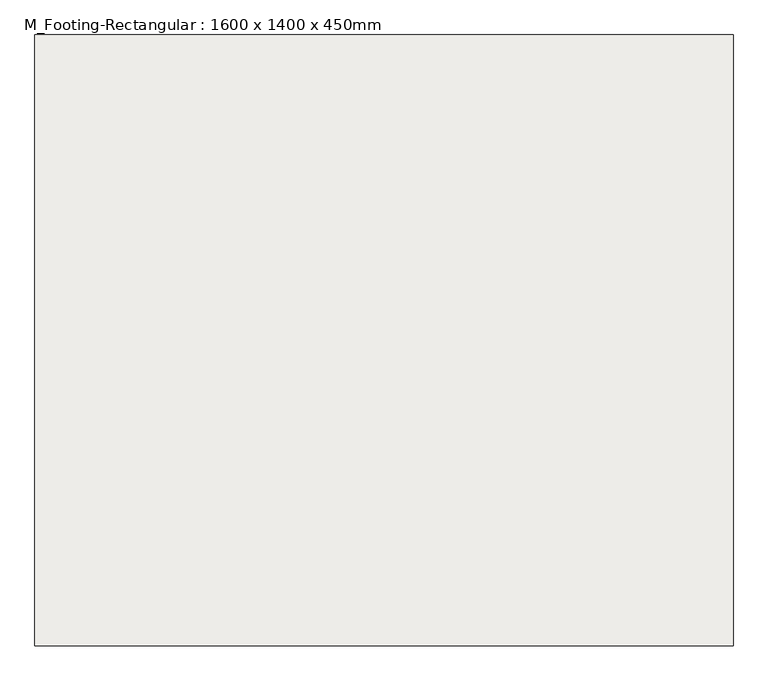
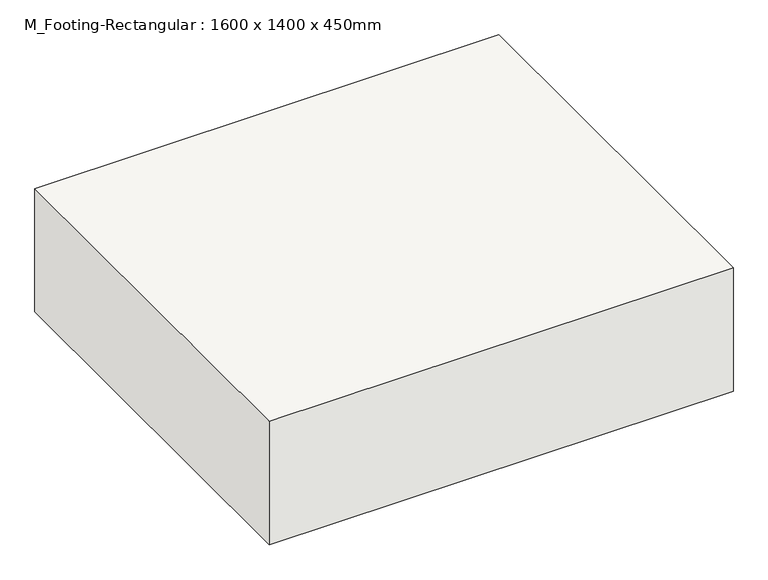
"""IFC4 building model written with IfcOpenShell, lengths in millimetres: slab geometry, M_Footing-Rectangular : 1600 x 1400 x 450mm."""

from ifc_helpers import new_model, si_unit, frame, origin, place, context, project, spatial, polyline, outline, extrude, source, transform, mapped, element, save


def m_footing_rectangular_1600_x_1400_x_450mm_70e385b2(model_context):
    return source(origin(), model_context, "Body", "SweptSolid", [
        extrude(outline(polyline([(800.0, 700.0), (800.0, -700.0), (-800.0, -700.0), (-800.0, 700.0), (800.0, 700.0)])), frame((0.0, 0.0, -450.0), z_axis=(0.0, 0.0, 1.0), x_axis=(1.0, 0.0, 0.0)), (0.0, 0.0, 1.0), 450.0),
    ])


if __name__ == "__main__":
    model = new_model("IFC4")
    model_context = context("Model", 3, world=origin())
    ifc_project = project(units=[si_unit("LENGTHUNIT", "METRE", prefix="MILLI")], contexts=[model_context])
    site = spatial("IfcSite", under=ifc_project)
    building = spatial("IfcBuilding", under=site)
    placement = place(None, origin())
    m_footing_rectangular_1600_x_1400_x_450mm_shape = m_footing_rectangular_1600_x_1400_x_450mm_70e385b2(model_context)
    element("IfcSlab", 1, ObjectType="M_Footing-Rectangular : 1600 x 1400 x 450mm", at=placement, inside=building, context=model_context, shape_type="MappedRepresentation", body=[
        mapped(m_footing_rectangular_1600_x_1400_x_450mm_shape, transform((0.0, 0.0, 0.0), x_axis=(1.0, 0.0, 0.0), y_axis=(0.0, 1.0, 0.0), z_axis=(0.0, 0.0, 1.0))),
    ])
    save(model, "model.ifc")

# Revit data of these elements
# Type "M_Footing-Rectangular : 1600 x 1400 x 450mm"
#   Width = 5' - 2.99213"
#   Length = 4' - 7.11811"
#   Foundation Thickness = 1' - 5.71654"
#   Structural Material [instance default] = Concrete, Cast-in-Place gray
#   Assembly Code = ""
# Element 1 (IfcSlab, "M_Footing-Rectangular : 1600 x 1400 x 450mm")
#   Materials on its faces: "Concrete, Cast-in-Place gray"
# Materials
#   "Concrete, Cast-in-Place gray": class "Concrete", colour RGB 192 192 192, transparency 0, Description = "Cast-in-place concrete", Cost = 0
